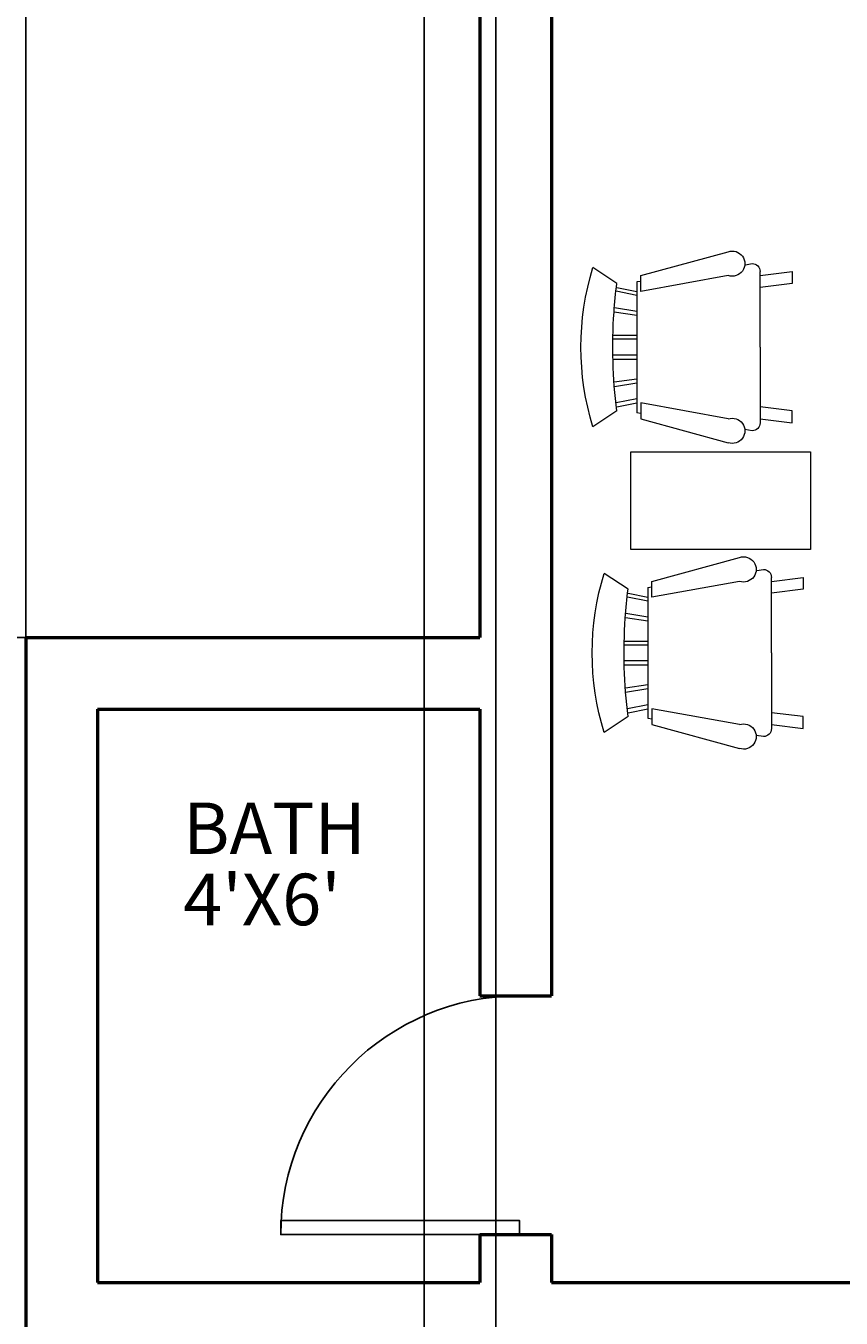
# Model space of a CAD drawing. Units: inches. Extents: x 5375 to 6084, y 16106 to 17259.
# Tile 16 of 32: x 5471 to 5573, y 16518 to 16680. Entities that reach past the tile are written whole.
import ezdxf

# ---------------------------------------------------------------- set-up
doc = ezdxf.new("R2010")
doc.units = ezdxf.units.IN
for name, color, linetype, lineweight in [('A-ANNO-DIMS', 2, 'Continuous', 18), ('A-AREA-IDEN', 5, 'Continuous', 18), ('DOOR', 4, 'Continuous', 25), ('FURNITURE', 3, 'Continuous', 18), ('WALL', 6, 'Continuous', 50)]:
    doc.layers.add(name, color=color, linetype=linetype, lineweight=lineweight)
doc.styles.get("Standard").update_dxf_attribs({"font": 'arial.ttf'})
doc.dimstyles.get("Standard").update_dxf_attribs({"dimtxt": 0.18, "dimasz": 0.18, "dimexe": 0.18, "dimexo": 0.0625, "dimgap": 0.09, "dimtad": 0, "dimtih": 1, "dimtoh": 1, "dimdec": 4, "dimzin": 0, "dimdsep": 46, "dimtxsty": 'Standard', "dimcen": 0.09, "dimadec": 0, "dimazin": 0, "dimtfac": 1, "dimtdec": 4, "dimtofl": 0, "dimtmove": 0, "dimatfit": 3, "dimfxl": 1, "dimtolj": 1, "dimtzin": 0, "dimarcsym": 0})

# ---------------------------------------------------------------- blocks, each defined once
blk = doc.blocks.new('*U2')
for p, q in [((0, 0), (0, -100)), ((750, 0), (750, -100))]:
    blk.add_line(p, q)
blk.add_lwpolyline([(0, 0), (0, 750), (43.75, 750), (43.75, 0)], close=True)
blk.add_arc((0, 0), 750, 0, 90)
blk = doc.blocks.new('Chair - Rocking')
for p, q in [((-8, -4.5), (-10, -1.5)), ((8, -4.5), (10, -1.5)), ((-7.5, -4.5), (-7, -7)), ((-6.5, -7), (-7.02225, -4.43)), ((-4.5, -7), (-4.96674, -4.19951)), ((-4, -7), (-4.40532, -4.16272)), ((-1.5, -4.05012), (-1.5, -7)), ((-1, -7), (-1, -4.05012)), ((1, -7), (1, -4.04655)), ((1.5, -4.05012), (1.5, -7)), ((4, -7), (4.40187, -4.18694)), ((4.5, -7), (4.96761, -4.19437)), ((6.5, -7), (7, -4.4057)), ((7.5, -4.5), (7, -7)), ((-9, -7.5), (-12, -18.49999)), ((-7, -7.5), (-9, -7.5)), ((-9, -18.49999), (-7, -7.5)), ((-8.23428, -6.99939), (-8.3093, -7.47958)), ((-8.23041, -7), (8.23915, -7)), ((7, -7.5), (9, -7.5)), ((9, -18.49999), (7, -7.5)), ((8.31071, -7.48854), (8.23449, -7.00073)), ((9, -7.5), (12, -18.49999)), ((-10.36644, -20.64523), (-10.5, -21.49999)), ((10.5, -21.49999), (10.3575, -20.58798)), ((-9, -22.49999), (-9.5, -26.49999)), ((0, -22.49999), (-9.5, -22.49999)), ((-8, -26.49999), (-7.5, -22.49999)), ((0, -22.49999), (9.5, -22.49999)), ((8, -26.49999), (7.5, -22.49999)), ((9, -22.49999), (9.5, -26.49999)), ((-9.5, -26.49999), (-8, -26.49999)), ((9.5, -26.49999), (8, -26.49999))]:
    blk.add_line(p, q)
for centre, radius, start, end in [((0, -34.08333), 34.08333, 72.93847, 107.0615), ((0, -68.25004), 64.25, 93.92211, 97.15267), ((0, -68.25004), 64.25, 82.84733, 93.92211), ((-10.5, -18.99999), 1.58114, 161.5651, 18.43495), ((10.5, -18.99999), 1.58114, 161.5651, 18.43495), ((-9.5, -21.49999), 1, 180, 270), ((9.5, -21.49999), 1, 270, 0)]:
    blk.add_arc(centre, radius, start, end)
blk = doc.blocks.new('*D35')
at = {"layer": 'A-ANNO-DIMS', "color": 0, "lineweight": -2, "transparency": 16777216}
for p, q in [((5527.56, 16699.58), (5375.56, 16699.58)), ((5375.74, 16699.4), (5375.74, 16651.76)), ((5375.74, 16603.76), (5375.74, 16651.4)), ((5527.56, 16603.58), (5375.56, 16603.58))]:
    blk.add_line(p, q, dxfattribs=at)
at = {"layer": 'A-ANNO-DIMS', "color": 0, "transparency": 16777216}
for points in [[(5375.71, 16699.4), (5375.77, 16699.4), (5375.74, 16699.58)], [(5375.71, 16603.76), (5375.77, 16603.76), (5375.74, 16603.58)]]:
    blk.add_solid(points, dxfattribs=at)
at = {"layer": 'Defpoints', "color": 0, "transparency": 16777216}
for p in [(5375.74, 16699.58), (5527.62, 16699.58), (5527.62, 16603.58)]:
    blk.add_point(p, dxfattribs=at)
at = {"layer": 'A-ANNO-DIMS', "color": 0, "transparency": 16777216, "insert": (5375.74, 16651.58), "char_height": 0.18, "attachment_point": 5}
blk.add_mtext('\\A1;96', dxfattribs=at)
blk = doc.blocks.new('*D40')
at = {"layer": 'A-ANNO-DIMS', "color": 0, "lineweight": -2, "transparency": 16777216}
for p, q in [((5529.62, 16876.52), (5529.62, 16106.48)), ((5520.62, 16867.52), (5520.62, 16106.48)), ((5520.8, 16106.66), (5524.97, 16106.66)), ((5529.44, 16106.66), (5525.27, 16106.66))]:
    blk.add_line(p, q, dxfattribs=at)
at = {"layer": 'A-ANNO-DIMS', "color": 0, "transparency": 16777216}
for points in [[(5520.8, 16106.69), (5520.8, 16106.63), (5520.62, 16106.66)], [(5529.44, 16106.69), (5529.44, 16106.63), (5529.62, 16106.66)]]:
    blk.add_solid(points, dxfattribs=at)
at = {"layer": 'Defpoints', "color": 0, "transparency": 16777216}
for p in [(5529.62, 16876.58), (5520.62, 16867.58), (5529.62, 16106.66)]:
    blk.add_point(p, dxfattribs=at)
at = {"layer": 'A-ANNO-DIMS', "color": 0, "transparency": 16777216, "insert": (5525.12, 16106.66), "char_height": 0.18, "attachment_point": 5}
blk.add_mtext('\\A1;9', dxfattribs=at)
blk = doc.blocks.new('*D47')
at = {"layer": 'A-ANNO-DIMS', "color": 0, "lineweight": -2, "transparency": 16777216}
for p, q in [((5470.62, 16603.64), (5470.62, 17259.16)), ((5470.8, 17258.98), (5495.4, 17258.98)), ((5520.44, 17258.98), (5495.84, 17258.98)), ((5520.62, 17206.64), (5520.62, 17259.16))]:
    blk.add_line(p, q, dxfattribs=at)
at = {"layer": 'A-ANNO-DIMS', "color": 0, "transparency": 16777216}
for points in [[(5470.8, 17259.01), (5470.8, 17258.95), (5470.62, 17258.98)], [(5520.44, 17259.01), (5520.44, 17258.95), (5520.62, 17258.98)]]:
    blk.add_solid(points, dxfattribs=at)
at = {"layer": 'Defpoints', "color": 0, "transparency": 16777216}
for p in [(5520.62, 17258.98), (5520.62, 17206.58), (5470.62, 16603.58)]:
    blk.add_point(p, dxfattribs=at)
at = {"layer": 'A-ANNO-DIMS', "color": 0, "transparency": 16777216, "insert": (5495.62, 17258.98), "char_height": 0.18, "attachment_point": 5}
blk.add_mtext('\\A1;50', dxfattribs=at)

msp = doc.modelspace()

# ---------------------------------------------------------------- linework, layer by layer
at = {"layer": 'FURNITURE'}
msp.add_lwpolyline([(5546.5804, 16626.903), (5569.1284, 16626.903), (5569.1284, 16614.6633), (5546.5804, 16614.6633)], close=True, dxfattribs=at)
at = {"layer": 'WALL'}
for p, q in [((5527.6199, 16699.5793), (5527.6199, 16603.5793)), ((5536.6199, 16690.5793), (5536.6199, 16558.5793)), ((5470.6199, 16603.5793), (5470.6199, 16212.3785)), ((5470.6199, 16603.5793), (5527.6199, 16603.5793)), ((5479.6199, 16594.5793), (5479.6199, 16522.5793)), ((5479.6199, 16594.5793), (5527.6199, 16594.5793)), ((5527.6199, 16594.5793), (5527.6199, 16558.5793)), ((5527.6199, 16558.5793), (5536.6199, 16558.5793)), ((5527.6199, 16528.5793), (5536.6199, 16528.5793)), ((5527.6199, 16528.5793), (5527.6199, 16522.5793)), ((5536.6199, 16528.5793), (5536.6199, 16522.5793)), ((5479.6199, 16522.5793), (5527.6199, 16522.5793)), ((5536.6199, 16522.5793), (5698.6199, 16522.5793))]:
    msp.add_line(p, q, dxfattribs=at)

# ---------------------------------------------------------------- block references
at = {"layer": 'DOOR', "xscale": 0.0399999999999999, "yscale": 0.0399999999999999, "zscale": 0.0399999999999999, "rotation": 90}
msp.add_blockref('*U2', (5532.6199, 16528.5793), dxfattribs=at)
at = {"layer": 'FURNITURE', "xscale": -1, "rotation": 90}
for p in [(5540.3202, 16640.0654), (5541.7377, 16601.6477)]:
    msp.add_blockref('Chair - Rocking', p, dxfattribs=at)

# ---------------------------------------------------------------- texts
at = {"layer": 'A-AREA-IDEN'}
for s, p in [('BATH', (5490.3775, 16576.3738)), ("4'X6'", (5490.3775, 16567.4407))]:
    msp.add_text(s, height=6.47981, dxfattribs=at).set_placement(p)

# ---------------------------------------------------------------- dimensions: what is measured, and where the dimension line sits
at = {"layer": 'A-ANNO-DIMS'}
for base, p1, p2, picture, middle in [((5520.6199, 17258.9793), (5470.6199, 16603.5793), (5520.6199, 17206.5793), '*D47', (5495.6199, 17258.9793)), ((5529.6199, 16106.6631), (5520.6199, 16867.5793), (5529.6199, 16876.5793), '*D40', (5525.1199, 16106.6631))]:
    dim = msp.add_linear_dim(base=base, p1=p1, p2=p2, dimstyle='Standard', override={"dimdec": 0, "dimlfac": 1, "dimrnd": 0, "dimzin": 0, "dimdsep": 46, "dimlunit": 2}, dxfattribs=at)
    dim.commit()
    dim.dimension.update_dxf_attribs({"geometry": picture, "text_midpoint": middle})
dim = msp.add_linear_dim(base=(5375.7423, 16699.5793), p1=(5527.6199, 16603.5793), p2=(5527.6199, 16699.5793), angle=90, dimstyle='Standard', override={"dimdec": 0, "dimlfac": 1, "dimrnd": 0, "dimzin": 0, "dimdsep": 46, "dimlunit": 2}, dxfattribs=at)
dim.commit()
dim.dimension.update_dxf_attribs({"geometry": '*D35', "text_midpoint": (5375.7423, 16651.5793)})

doc.saveas('drawing.dxf')
